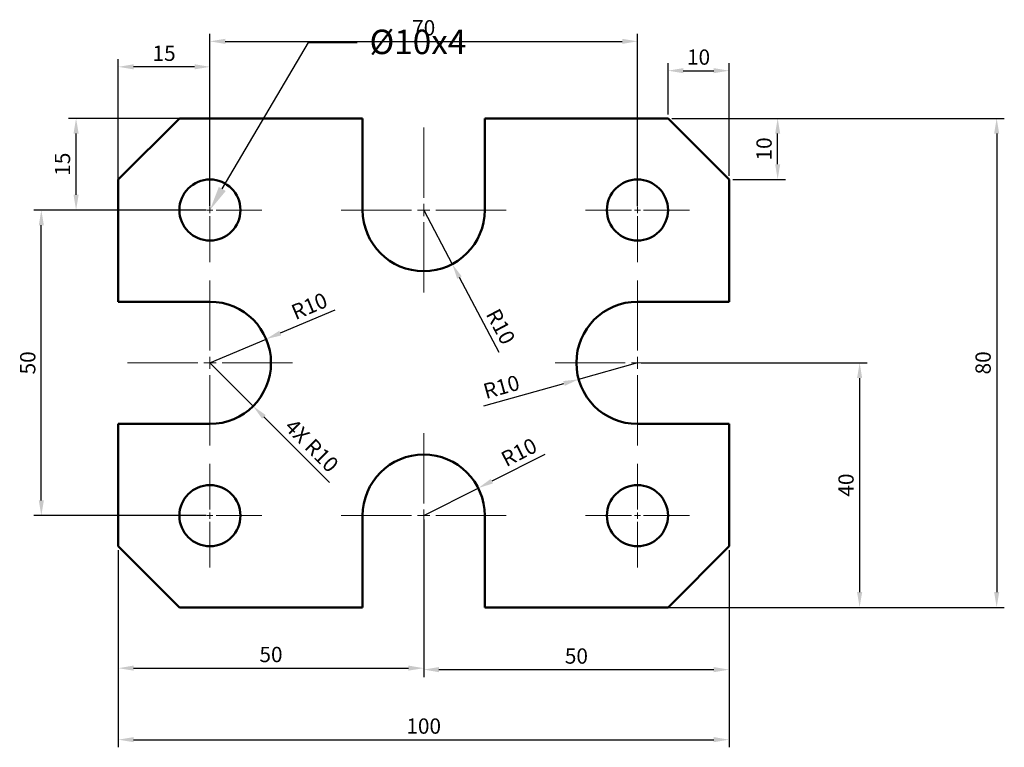
# Model space of a CAD drawing. Units: millimetres. Extents: x -16 to 145, y -23 to 96.
import ezdxf
from ezdxf import colors
from ezdxf.entities.mleader import LeaderData, LeaderLine
from ezdxf.math import Vec2, Vec3

# ---------------------------------------------------------------- set-up
doc = ezdxf.new("R2010")
doc.units = ezdxf.units.MM
doc.linetypes.add('CENTER2', pattern=[28.575, 19.05, -3.175, 3.175, -3.175])
for name, color, linetype, lineweight in [('M-CNTR', 4, 'CENTER2', 18), ('M-CONS', 8, 'Continuous', 13), ('M-DIMS', 2, 'Continuous', 25), ('M-OUTL', 7, 'Continuous', 50)]:
    doc.layers.add(name, color=color, linetype=linetype, lineweight=lineweight)
doc.styles.get("Standard").update_dxf_attribs({"font": 'arial.ttf'})
doc.dimstyles.new('ISO-25', dxfattribs={"dimtxt": 2.5, "dimasz": 2.5, "dimexe": 1.2505, "dimexo": 0.625, "dimtad": 1, "dimtxsty": 'Standard', "dimcen": 2.5, "dimadec": 0, "dimazin": 0, "dimtfac": 1, "dimtmove": 0, "dimatfit": 3, "dimfxl": 1, "dimarcsym": 0})

# ---------------------------------------------------------------- blocks, each defined once
blk = doc.blocks.new('*U1')
at = {"layer": 'M-CNTR', "color": 0, "transparency": 16777216}
for p, q in [((0, 1), (0, 8.5)), ((-8.5, 0), (-1, 0)), ((1, 0), (8.5, 0)), ((0, -8.5), (0, -1))]:
    blk.add_line(p, q, dxfattribs=at)
at = {"layer": 'M-CNTR', "color": 0, "linetype": 'Continuous', "transparency": 16777216}
for p, q in [((-0.5, 0), (0.5, 0)), ((0, -0.5), (0, 0.5))]:
    blk.add_line(p, q, dxfattribs=at)
blk = doc.blocks.new('*U2')
at = {"layer": 'M-CNTR', "color": 0, "transparency": 16777216}
for p, q in [((0, 1), (0, 8.5)), ((-8.5, 0), (-1, 0)), ((1, 0), (8.5, 0)), ((0, -8.5), (0, -1))]:
    blk.add_line(p, q, dxfattribs=at)
at = {"layer": 'M-CNTR', "color": 0, "linetype": 'Continuous', "transparency": 16777216}
for p, q in [((-0.5, 0), (0.5, 0)), ((0, -0.5), (0, 0.5))]:
    blk.add_line(p, q, dxfattribs=at)
blk = doc.blocks.new('*U3')
at = {"layer": 'M-CNTR', "color": 0, "transparency": 16777216}
for p, q in [((0, 1), (0, 8.5)), ((-8.5, 0), (-1, 0)), ((1, 0), (8.5, 0)), ((0, -8.5), (0, -1))]:
    blk.add_line(p, q, dxfattribs=at)
at = {"layer": 'M-CNTR', "color": 0, "linetype": 'Continuous', "transparency": 16777216}
for p, q in [((-0.5, 0), (0.5, 0)), ((0, -0.5), (0, 0.5))]:
    blk.add_line(p, q, dxfattribs=at)
blk = doc.blocks.new('*U4')
at = {"layer": 'M-CNTR', "color": 0, "transparency": 16777216}
for p, q in [((0, 1), (0, 8.5)), ((-8.5, 0), (-1, 0)), ((1, 0), (8.5, 0)), ((0, -8.5), (0, -1))]:
    blk.add_line(p, q, dxfattribs=at)
at = {"layer": 'M-CNTR', "color": 0, "linetype": 'Continuous', "transparency": 16777216}
for p, q in [((-0.5, 0), (0.5, 0)), ((0, -0.5), (0, 0.5))]:
    blk.add_line(p, q, dxfattribs=at)
blk = doc.blocks.new('*U5')
at = {"layer": 'M-CNTR', "color": 0, "transparency": 16777216}
for p, q in [((0, 2), (0, 13.5)), ((-13.5, 0), (-2, 0)), ((2, 0), (13.5, 0)), ((0, -13.5), (0, -2))]:
    blk.add_line(p, q, dxfattribs=at)
at = {"layer": 'M-CNTR', "color": 0, "linetype": 'Continuous', "transparency": 16777216}
for p, q in [((-1, 0), (1, 0)), ((0, -1), (0, 1))]:
    blk.add_line(p, q, dxfattribs=at)
blk = doc.blocks.new('*U6')
at = {"layer": 'M-CNTR', "color": 0, "transparency": 16777216}
for p, q in [((0, 2), (0, 13.5)), ((-13.5, 0), (-2, 0)), ((2, 0), (13.5, 0)), ((0, -13.5), (0, -2))]:
    blk.add_line(p, q, dxfattribs=at)
at = {"layer": 'M-CNTR', "color": 0, "linetype": 'Continuous', "transparency": 16777216}
for p, q in [((-1, 0), (1, 0)), ((0, -1), (0, 1))]:
    blk.add_line(p, q, dxfattribs=at)
blk = doc.blocks.new('*U7')
at = {"layer": 'M-CNTR', "color": 0, "transparency": 16777216}
for p, q in [((0, 2), (0, 13.5)), ((-13.5, 0), (-2, 0)), ((2, 0), (13.5, 0)), ((0, -13.5), (0, -2))]:
    blk.add_line(p, q, dxfattribs=at)
at = {"layer": 'M-CNTR', "color": 0, "linetype": 'Continuous', "transparency": 16777216}
for p, q in [((-1, 0), (1, 0)), ((0, -1), (0, 1))]:
    blk.add_line(p, q, dxfattribs=at)
blk = doc.blocks.new('*U8')
at = {"layer": 'M-CNTR', "color": 0, "transparency": 16777216}
for p, q in [((0, 2), (0, 13.5)), ((-13.5, 0), (-2, 0)), ((2, 0), (13.5, 0)), ((0, -13.5), (0, -2))]:
    blk.add_line(p, q, dxfattribs=at)
at = {"layer": 'M-CNTR', "color": 0, "linetype": 'Continuous', "transparency": 16777216}
for p, q in [((-1, 0), (1, 0)), ((0, -1), (0, 1))]:
    blk.add_line(p, q, dxfattribs=at)
blk = doc.blocks.new('*D9')
at = {"layer": 'Defpoints', "color": 0, "transparency": 16777216}
for p in [(0, 88.43), (0, 65), (15, 65)]:
    blk.add_point(p, dxfattribs=at)
at = {"layer": 'M-DIMS', "color": 0, "lineweight": -2, "transparency": 16777216}
for p, q in [((0, 65.62), (0, 89.68)), ((15, 65.62), (15, 89.68)), ((12.5, 88.43), (2.5, 88.43))]:
    blk.add_line(p, q, dxfattribs=at)
at = {"layer": 'M-DIMS', "color": 0, "transparency": 16777216}
for points in [[(2.5, 88.85), (2.5, 88.02), (0, 88.43)], [(12.5, 88.85), (12.5, 88.02), (15, 88.43)]]:
    blk.add_solid(points, dxfattribs=at)
at = {"layer": 'M-DIMS', "color": 0, "transparency": 16777216, "insert": (7.5, 90.33), "char_height": 2.5, "attachment_point": 5}
blk.add_mtext('15', dxfattribs=at)
blk = doc.blocks.new('*D10')
at = {"layer": 'Defpoints', "color": 0, "transparency": 16777216}
for p in [(-6.91, 80), (15, 80), (15, 65)]:
    blk.add_point(p, dxfattribs=at)
at = {"layer": 'M-DIMS', "color": 0, "lineweight": -2, "transparency": 16777216}
for p, q in [((14.38, 80), (-8.16, 80)), ((-6.91, 67.5), (-6.91, 77.5)), ((14.38, 65), (-8.16, 65))]:
    blk.add_line(p, q, dxfattribs=at)
at = {"layer": 'M-DIMS', "color": 0, "transparency": 16777216}
for points in [[(-7.33, 77.5), (-6.49, 77.5), (-6.91, 80)], [(-7.33, 67.5), (-6.49, 67.5), (-6.91, 65)]]:
    blk.add_solid(points, dxfattribs=at)
at = {"layer": 'M-DIMS', "color": 0, "transparency": 16777216, "insert": (-8.81, 72.5), "char_height": 2.5, "attachment_point": 5, "rotation": 90}
blk.add_mtext('15', dxfattribs=at)
blk = doc.blocks.new('*D11')
at = {"layer": 'Defpoints', "color": 0, "transparency": 16777216}
for p in [(0, 10), (100, 10), (100, -21.65)]:
    blk.add_point(p, dxfattribs=at)
at = {"layer": 'M-DIMS', "color": 0, "lineweight": -2, "transparency": 16777216}
for p, q in [((0, 9.38), (0, -22.9)), ((100, 9.38), (100, -22.9)), ((2.5, -21.65), (97.5, -21.65))]:
    blk.add_line(p, q, dxfattribs=at)
at = {"layer": 'M-DIMS', "color": 0, "transparency": 16777216}
for points in [[(2.5, -21.23), (2.5, -22.06), (0, -21.65)], [(97.5, -21.23), (97.5, -22.06), (100, -21.65)]]:
    blk.add_solid(points, dxfattribs=at)
at = {"layer": 'M-DIMS', "color": 0, "transparency": 16777216, "insert": (50, -19.75), "char_height": 2.5, "attachment_point": 5}
blk.add_mtext('100', dxfattribs=at)
blk = doc.blocks.new('*D12')
at = {"layer": 'Defpoints', "color": 0, "transparency": 16777216}
for p in [(50, 15), (0, 10), (50, -9.95)]:
    blk.add_point(p, dxfattribs=at)
at = {"layer": 'M-DIMS', "color": 0, "lineweight": -2, "transparency": 16777216}
for p, q in [((50, 14.38), (50, -11.2)), ((0, 9.38), (0, -11.2)), ((2.5, -9.95), (47.5, -9.95))]:
    blk.add_line(p, q, dxfattribs=at)
at = {"layer": 'M-DIMS', "color": 0, "transparency": 16777216}
for points in [[(2.5, -9.53), (2.5, -10.36), (0, -9.95)], [(47.5, -9.53), (47.5, -10.36), (50, -9.95)]]:
    blk.add_solid(points, dxfattribs=at)
at = {"layer": 'M-DIMS', "color": 0, "transparency": 16777216, "insert": (25, -8.04), "char_height": 2.5, "attachment_point": 5}
blk.add_mtext('50', dxfattribs=at)
blk = doc.blocks.new('*D13')
at = {"layer": 'Defpoints', "color": 0, "transparency": 16777216}
for p in [(50, 15), (100, 10), (100, -10.19)]:
    blk.add_point(p, dxfattribs=at)
at = {"layer": 'M-DIMS', "color": 0, "lineweight": -2, "transparency": 16777216}
for p, q in [((50, 14.38), (50, -11.44)), ((100, 9.38), (100, -11.44)), ((52.5, -10.19), (97.5, -10.19))]:
    blk.add_line(p, q, dxfattribs=at)
at = {"layer": 'M-DIMS', "color": 0, "transparency": 16777216}
for points in [[(52.5, -9.77), (52.5, -10.61), (50, -10.19)], [(97.5, -9.77), (97.5, -10.61), (100, -10.19)]]:
    blk.add_solid(points, dxfattribs=at)
at = {"layer": 'M-DIMS', "color": 0, "transparency": 16777216, "insert": (75, -8.29), "char_height": 2.5, "attachment_point": 5}
blk.add_mtext('50', dxfattribs=at)
blk = doc.blocks.new('*D14')
at = {"layer": 'Defpoints', "color": 0, "transparency": 16777216}
for p in [(90, 80), (90, 0), (143.81, 0)]:
    blk.add_point(p, dxfattribs=at)
at = {"layer": 'M-DIMS', "color": 0, "lineweight": -2, "transparency": 16777216}
for p, q in [((90.63, 80), (145.06, 80)), ((143.81, 77.5), (143.81, 2.5)), ((90.63, 0), (145.06, 0))]:
    blk.add_line(p, q, dxfattribs=at)
at = {"layer": 'M-DIMS', "color": 0, "transparency": 16777216}
for points in [[(143.39, 77.5), (144.22, 77.5), (143.81, 80)], [(143.39, 2.5), (144.22, 2.5), (143.81, 0)]]:
    blk.add_solid(points, dxfattribs=at)
at = {"layer": 'M-DIMS', "color": 0, "transparency": 16777216, "insert": (141.91, 40), "char_height": 2.5, "attachment_point": 5, "rotation": 90}
blk.add_mtext('80', dxfattribs=at)
blk = doc.blocks.new('*D15')
at = {"layer": 'Defpoints', "color": 0, "transparency": 16777216}
for p in [(85, 40), (85, 0), (121.37, 0)]:
    blk.add_point(p, dxfattribs=at)
at = {"layer": 'M-DIMS', "color": 0, "lineweight": -2, "transparency": 16777216}
for p, q in [((85.62, 40), (122.62, 40)), ((121.37, 37.5), (121.37, 2.5)), ((85.62, 0), (122.62, 0))]:
    blk.add_line(p, q, dxfattribs=at)
at = {"layer": 'M-DIMS', "color": 0, "transparency": 16777216}
for points in [[(120.95, 37.5), (121.79, 37.5), (121.37, 40)], [(120.95, 2.5), (121.79, 2.5), (121.37, 0)]]:
    blk.add_solid(points, dxfattribs=at)
at = {"layer": 'M-DIMS', "color": 0, "transparency": 16777216, "insert": (119.47, 20), "char_height": 2.5, "attachment_point": 5, "rotation": 90}
blk.add_mtext('40', dxfattribs=at)
blk = doc.blocks.new('*D16')
at = {"layer": 'Defpoints', "color": 0, "transparency": 16777216}
for p in [(100, 80), (107.95, 80), (100, 70)]:
    blk.add_point(p, dxfattribs=at)
at = {"layer": 'M-DIMS', "color": 0, "lineweight": -2, "transparency": 16777216}
for p, q in [((100.62, 80), (109.21, 80)), ((107.95, 72.5), (107.95, 77.5)), ((100.62, 70), (109.21, 70))]:
    blk.add_line(p, q, dxfattribs=at)
at = {"layer": 'M-DIMS', "color": 0, "transparency": 16777216}
for points in [[(107.54, 77.5), (108.37, 77.5), (107.95, 80)], [(107.54, 72.5), (108.37, 72.5), (107.95, 70)]]:
    blk.add_solid(points, dxfattribs=at)
at = {"layer": 'M-DIMS', "color": 0, "transparency": 16777216, "insert": (106.05, 75), "char_height": 2.5, "attachment_point": 5, "rotation": 90}
blk.add_mtext('10', dxfattribs=at)
blk = doc.blocks.new('*D17')
at = {"layer": 'Defpoints', "color": 0, "transparency": 16777216}
for p in [(100, 87.8), (90, 80), (100, 70)]:
    blk.add_point(p, dxfattribs=at)
at = {"layer": 'M-DIMS', "color": 0, "lineweight": -2, "transparency": 16777216}
for p, q in [((90, 80.62), (90, 89.05)), ((100, 70.62), (100, 89.05)), ((92.5, 87.8), (97.5, 87.8))]:
    blk.add_line(p, q, dxfattribs=at)
at = {"layer": 'M-DIMS', "color": 0, "transparency": 16777216}
for points in [[(92.5, 88.22), (92.5, 87.39), (90, 87.8)], [(97.5, 88.22), (97.5, 87.39), (100, 87.8)]]:
    blk.add_solid(points, dxfattribs=at)
at = {"layer": 'M-DIMS', "color": 0, "transparency": 16777216, "insert": (95, 89.7), "char_height": 2.5, "attachment_point": 5}
blk.add_mtext('10', dxfattribs=at)
blk = doc.blocks.new('*D18')
at = {"layer": 'Defpoints', "color": 0, "transparency": 16777216}
for p in [(50, 65), (54.68, 56.16)]:
    blk.add_point(p, dxfattribs=at)
at = {"layer": 'M-DIMS', "color": 0, "lineweight": -2, "transparency": 16777216}
for p, q in [((50, 65), (54.68, 56.16)), ((62.33, 41.71), (55.85, 53.95))]:
    blk.add_line(p, q, dxfattribs=at)
at = {"layer": 'M-DIMS', "color": 0, "transparency": 16777216}
blk.add_solid([(56.22, 54.15), (55.48, 53.76), (54.68, 56.16)], dxfattribs=at)
at = {"layer": 'M-DIMS', "color": 0, "transparency": 16777216, "insert": (62.32, 45.79), "char_height": 2.5, "attachment_point": 5, "rotation": 297.8929}
blk.add_mtext('R10', dxfattribs=at)
blk = doc.blocks.new('*D19')
at = {"layer": 'Defpoints', "color": 0, "transparency": 16777216}
for p in [(24.21, 43.89), (15, 40)]:
    blk.add_point(p, dxfattribs=at)
at = {"layer": 'M-DIMS', "color": 0, "lineweight": -2, "transparency": 16777216}
for p, q in [((35.46, 48.64), (26.51, 44.86)), ((15, 40), (24.21, 43.89))]:
    blk.add_line(p, q, dxfattribs=at)
at = {"layer": 'M-DIMS', "color": 0, "transparency": 16777216}
blk.add_solid([(26.35, 45.25), (26.68, 44.48), (24.21, 43.89)], dxfattribs=at)
at = {"layer": 'M-DIMS', "color": 0, "transparency": 16777216, "insert": (31.4, 48.99), "char_height": 2.5, "attachment_point": 5, "rotation": 22.8987}
blk.add_mtext('R10', dxfattribs=at)
blk = doc.blocks.new('*D20')
at = {"layer": 'Defpoints', "color": 0, "transparency": 16777216}
for p in [(58.93, 19.51), (50, 15)]:
    blk.add_point(p, dxfattribs=at)
at = {"layer": 'M-DIMS', "color": 0, "lineweight": -2, "transparency": 16777216}
for p, q in [((69.83, 25.02), (61.16, 20.64)), ((50, 15), (58.93, 19.51))]:
    blk.add_line(p, q, dxfattribs=at)
at = {"layer": 'M-DIMS', "color": 0, "transparency": 16777216}
blk.add_solid([(60.97, 21.01), (61.34, 20.27), (58.93, 19.51)], dxfattribs=at)
at = {"layer": 'M-DIMS', "color": 0, "transparency": 16777216, "insert": (65.75, 25.09), "char_height": 2.5, "attachment_point": 5, "rotation": 26.808}
blk.add_mtext('R10', dxfattribs=at)
blk = doc.blocks.new('*D21')
at = {"layer": 'Defpoints', "color": 0, "transparency": 16777216}
for p in [(85, 40), (75.37, 37.3)]:
    blk.add_point(p, dxfattribs=at)
at = {"layer": 'M-DIMS', "color": 0, "lineweight": -2, "transparency": 16777216}
for p, q in [((85, 40), (75.37, 37.3)), ((59.85, 32.96), (72.96, 36.63))]:
    blk.add_line(p, q, dxfattribs=at)
at = {"layer": 'M-DIMS', "color": 0, "transparency": 16777216}
blk.add_solid([(72.85, 37.03), (73.08, 36.23), (75.37, 37.3)], dxfattribs=at)
at = {"layer": 'M-DIMS', "color": 0, "transparency": 16777216, "insert": (62.81, 35.76), "char_height": 2.5, "attachment_point": 5, "rotation": 15.6409}
blk.add_mtext('R10', dxfattribs=at)
blk = doc.blocks.new('*D22')
at = {"layer": 'Defpoints', "color": 0, "transparency": 16777216}
for p in [(85, 92.6), (15, 65), (85, 65)]:
    blk.add_point(p, dxfattribs=at)
at = {"layer": 'M-DIMS', "color": 0, "lineweight": -2, "transparency": 16777216}
for p, q in [((15, 65.62), (15, 93.85)), ((85, 65.62), (85, 93.85)), ((17.5, 92.6), (82.5, 92.6))]:
    blk.add_line(p, q, dxfattribs=at)
at = {"layer": 'M-DIMS', "color": 0, "transparency": 16777216}
for points in [[(17.5, 93.02), (17.5, 92.18), (15, 92.6)], [(82.5, 93.02), (82.5, 92.18), (85, 92.6)]]:
    blk.add_solid(points, dxfattribs=at)
at = {"layer": 'M-DIMS', "color": 0, "transparency": 16777216, "insert": (50, 94.5), "char_height": 2.5, "attachment_point": 5}
blk.add_mtext('70', dxfattribs=at)
blk = doc.blocks.new('*D23')
at = {"layer": 'Defpoints', "color": 0, "transparency": 16777216}
for p in [(-12.6, 65), (15, 65), (15, 15)]:
    blk.add_point(p, dxfattribs=at)
at = {"layer": 'M-DIMS', "color": 0, "lineweight": -2, "transparency": 16777216}
for p, q in [((14.38, 65), (-13.85, 65)), ((-12.6, 17.5), (-12.6, 62.5)), ((14.38, 15), (-13.85, 15))]:
    blk.add_line(p, q, dxfattribs=at)
at = {"layer": 'M-DIMS', "color": 0, "transparency": 16777216}
for points in [[(-13.02, 62.5), (-12.18, 62.5), (-12.6, 65)], [(-13.02, 17.5), (-12.18, 17.5), (-12.6, 15)]]:
    blk.add_solid(points, dxfattribs=at)
at = {"layer": 'M-DIMS', "color": 0, "transparency": 16777216, "insert": (-14.5, 40), "char_height": 2.5, "attachment_point": 5, "rotation": 90}
blk.add_mtext('50', dxfattribs=at)
blk = doc.blocks.new('*D24')
at = {"layer": 'Defpoints', "color": 0, "transparency": 16777216}
for p in [(15, 40), (22.07, 32.93)]:
    blk.add_point(p, dxfattribs=at)
at = {"layer": 'M-DIMS', "color": 0, "lineweight": -2, "transparency": 16777216}
for p, q in [((15, 40), (22.07, 32.93)), ((34.58, 20.42), (23.84, 31.16))]:
    blk.add_line(p, q, dxfattribs=at)
at = {"layer": 'M-DIMS', "color": 0, "transparency": 16777216}
blk.add_solid([(24.13, 31.46), (23.54, 30.87), (22.07, 32.93)], dxfattribs=at)
at = {"layer": 'M-DIMS', "color": 0, "transparency": 16777216, "insert": (31.44, 26.25), "char_height": 2.5, "attachment_point": 5, "rotation": 315}
blk.add_mtext('4X R10', dxfattribs=at)

msp = doc.modelspace()

# ---------------------------------------------------------------- linework, layer by layer
at = {"layer": 'M-CONS'}
for p, q in [((50, 55), (50, 55)), ((25, 40), (25, 40)), ((75, 40), (75, 40)), ((50, 25), (50, 25))]:
    msp.add_line(p, q, dxfattribs=at)
at = {"layer": 'M-OUTL'}
for p, q in [((10, 80), (0, 70)), ((15, 80), (10, 80)), ((40, 80), (15, 80)), ((40, 65), (40, 80)), ((90, 80), (60, 80)), ((60, 80), (60, 65)), ((90, 80), (100, 70)), ((0, 70), (0, 50)), ((100, 50), (100, 70)), ((0, 50), (15, 50)), ((100, 50), (85, 50)), ((0, 30), (0, 10)), ((15, 30), (0, 30)), ((85, 30), (100, 30)), ((100, 10), (100, 30)), ((40, 15), (40, 0)), ((60, 0), (60, 15)), ((0, 10), (10, 0)), ((100, 10), (90, 0)), ((10, 0), (40, 0)), ((60, 0), (90, 0))]:
    msp.add_line(p, q, dxfattribs=at)
for centre in [(15, 65), (85, 65), (15, 15), (85, 15)]:
    msp.add_circle(centre, 5, dxfattribs=at)
for centre, start, end in [((50, 65), 180, 270), ((50, 65), 270, 0), ((15, 40), 0, 90), ((85, 40), 90, 180), ((15, 40), 270, 0), ((85, 40), 180, 270), ((50, 15), 90, 180), ((50, 15), 0, 90)]:
    msp.add_arc(centre, 10, start, end, dxfattribs=at)

# ---------------------------------------------------------------- block references
at = {"layer": 'M-CNTR'}
for name, p in [('*U7', (50, 65)), ('*U1', (15, 65)), ('*U2', (85, 65)), ('*U8', (15, 40)), ('*U6', (85, 40)), ('*U5', (50, 15)), ('*U3', (15, 15)), ('*U4', (85, 15))]:
    msp.add_blockref(name, p, dxfattribs=at)

# ---------------------------------------------------------------- dimensions: what is measured, and where the dimension line sits
at = {"layer": 'M-DIMS'}
for base, p1, p2, override, picture, middle in [((85, 92.6), (15, 65), (85, 65), {"dimdec": 0, "dimlfac": 1, "dimrnd": 0, "dimzin": 0, "dimdsep": 46, "dimlunit": 2}, '*D22', (50, 94.501)), ((0, 88.432), (15, 65), (0, 65), {"dimclrd": 0, "dimclre": 0, "dimclrt": 0}, '*D9', (7.5, 90.334)), ((100, 87.802), (90, 80), (100, 70), {"dimclrd": 0, "dimclre": 0, "dimclrt": 0}, '*D17', (95, 89.703)), ((50, -9.946), (0, 10), (50, 15), {"dimclrd": 0, "dimclre": 0, "dimclrt": 0}, '*D12', (25, -8.045)), ((100, -10.19), (50, 15), (100, 10), {"dimclrd": 0, "dimclre": 0, "dimclrt": 0}, '*D13', (75, -8.289)), ((100, -21.647), (0, 10), (100, 10), {"dimclrd": 0, "dimclre": 0, "dimclrt": 0}, '*D11', (50, -19.745))]:
    dim = msp.add_linear_dim(base=base, p1=p1, p2=p2, dimstyle='ISO-25', override=override, dxfattribs=at)
    dim.commit()
    dim.dimension.update_dxf_attribs({"geometry": picture, "text_midpoint": middle})
for base, p1, p2, override, picture, middle in [((-6.91, 80), (15, 65), (15, 80), {"dimclrd": 0, "dimclre": 0, "dimclrt": 0}, '*D10', (-8.811, 72.5)), ((143.807, 0), (90, 80), (90, 0), {"dimclrd": 0, "dimclre": 0, "dimclrt": 0}, '*D14', (141.905, 40)), ((107.955, 80.002), (100, 70), (100, 80.002), {"dimclrd": 0, "dimclre": 0, "dimclrt": 0}, '*D16', (106.053, 75.001)), ((-12.6, 65), (15, 15), (15, 65), {"dimdec": 0, "dimlfac": 1, "dimrnd": 0, "dimzin": 0, "dimdsep": 46, "dimlunit": 2}, '*D23', (-14.501, 40)), ((121.369, 0), (85, 40), (85, 0), {"dimclrd": 0, "dimclre": 0, "dimclrt": 0}, '*D15', (119.467, 20))]:
    dim = msp.add_linear_dim(base=base, p1=p1, p2=p2, angle=90, dimstyle='ISO-25', override=override, dxfattribs=at)
    dim.commit()
    dim.dimension.update_dxf_attribs({"geometry": picture, "text_midpoint": middle})
for center, mpoint, picture, middle in [((50, 65), (54.678, 56.162), '*D18', (60.639, 44.9)), ((85, 40), (75.37, 37.304), '*D21', (63.322, 33.931))]:
    dim = msp.add_radius_dim(center=center, mpoint=mpoint, dimstyle='ISO-25', override={"dimclrd": 0, "dimclre": 0, "dimclrt": 0}, dxfattribs=at)
    dim.commit()
    dim.dimension.update_dxf_attribs({"geometry": picture, "text_midpoint": middle, "dimtype": 164})
for center, mpoint, picture, middle in [((15, 40), (24.212, 43.891), '*D19', (31.401, 48.992)), ((50, 15), (58.925, 19.51), '*D20', (65.75, 25.089))]:
    dim = msp.add_radius_dim(center=center, mpoint=mpoint, dimstyle='ISO-25', override={"dimclrd": 0, "dimclre": 0, "dimclrt": 0}, dxfattribs=at)
    dim.commit()
    dim.dimension.update_dxf_attribs({"geometry": picture, "text_midpoint": middle})
dim = msp.add_radius_dim(center=(15, 40), mpoint=(22.071, 32.929), text='4X <>', dimstyle='ISO-25', override={"dimdec": 0, "dimlfac": 1, "dimrnd": 0, "dimzin": 0, "dimdsep": 46, "dimlunit": 2}, dxfattribs=at)
dim.commit()
dim.dimension.update_dxf_attribs({"geometry": '*D24', "text_midpoint": (31.437, 26.252)})

# ---------------------------------------------------------------- leaders
ml = msp.add_multileader_mtext('Standard', dxfattribs=at)
ml.set_content('%%C10x4', color=256)
ml.set_leader_properties()
ml.build(insert=Vec2(0, 0))
ctx = ml.context
ctx.base_point, ctx.plane_origin = Vec3(39.128, 92.433), Vec3(15, 65)
notes = []
notes.append((ctx, [(0, (1, 1, 0), (31.128, 92.433), (1, 0), 8, [(0, [(15, 65)], 0, [])])]))
ctx.mtext.insert, ctx.mtext.flow_direction = Vec3(41.128, 94.514), 5
for ctx, leaders in notes:
    for number, flags, end, landing, length, lines in leaders:
        leader = LeaderData()
        leader.index, (leader.has_last_leader_line, leader.has_dogleg_vector, leader.attachment_direction) = number, flags
        leader.last_leader_point, leader.dogleg_vector, leader.dogleg_length = Vec3(end), Vec3(landing), length
        for number, points, colour, breaks in lines:
            line = LeaderLine()
            line.index, line.vertices, line.color, line.breaks = number, Vec3.list(points), colors.encode_raw_color(colour), breaks
            leader.lines.append(line)
        ctx.leaders.append(leader)

doc.saveas('drawing.dxf')
